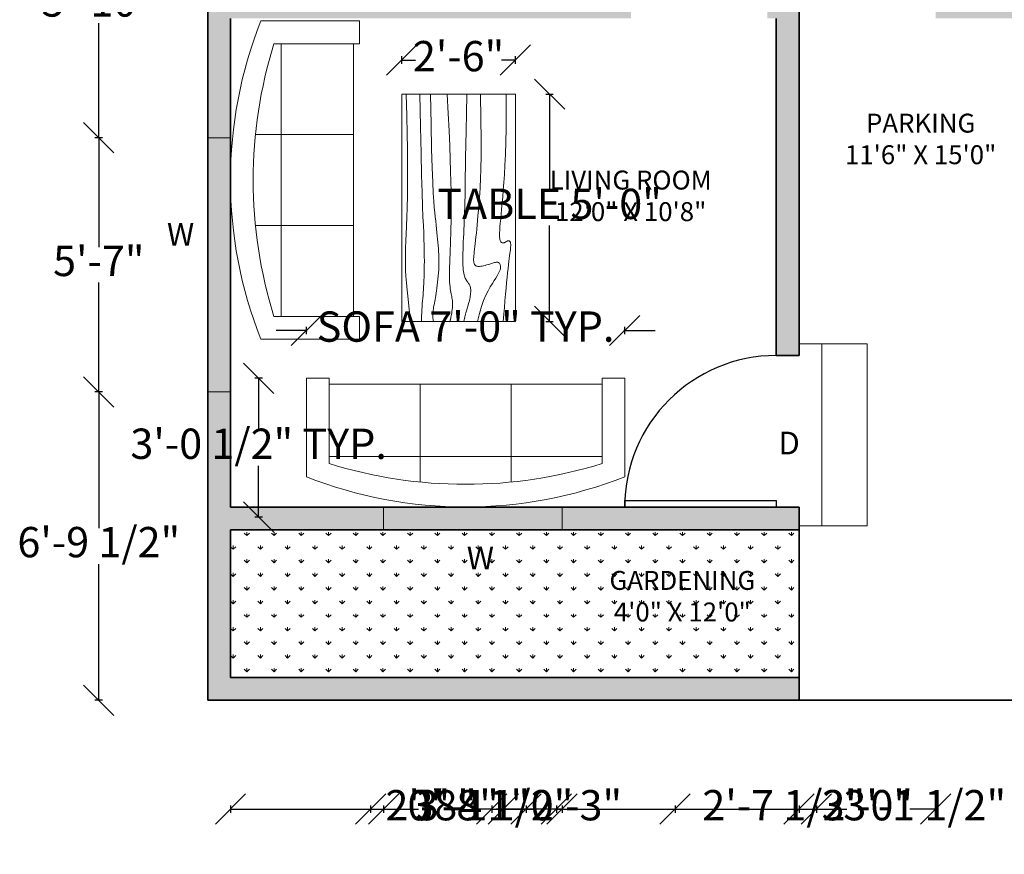
# Model space of a CAD drawing. Units: inches. Extents: x 2247 to 2713, y 588 to 1209.
# Tile 1 of 5: x 2314 to 2574, y 588 to 808. Entities that reach past the tile are written whole.
import ezdxf

# ---------------------------------------------------------------- set-up
doc = ezdxf.new("R2010")
doc.units = ezdxf.units.IN
for name, color, linetype, lineweight in [('A-ANNO-DIMS', 2, 'Continuous', 18), ('A-ANNO-TEXT', 7, 'Continuous', 18), ('A-AREA-IDEN', 7, 'Continuous', 25), ('A-DOOR', 3, 'Continuous', 25), ('A-FLOR-STRS', 7, 'Continuous', 18), ('A-FURN', 8, 'Continuous', 18), ('A-GLAZ', 4, 'Continuous', 18), ('A-GLAZ-PATT', 7, 'Continuous', 13), ('A-WALL', 7, 'Continuous', 35), ('A-WALL-PATT', 4, 'Continuous', 13)]:
    doc.layers.add(name, color=color, linetype=linetype, lineweight=lineweight)
doc.layers.add('L-PLNT-PATT', color=116, linetype='Continuous', lineweight=13, true_color=0x136734)
doc.styles.get("Standard").update_dxf_attribs({"font": 'arial.ttf'})
doc.dimstyles.new('ISO-25', dxfattribs={"dimtxt": 8, "dimasz": 8, "dimexe": 1, "dimexo": 1, "dimtad": 0, "dimtih": 1, "dimtoh": 1, "dimlunit": 3, "dimtxsty": 'Standard', "dimblk": 'OBLIQUE', "dimcen": 2.5, "dimadec": 0, "dimazin": 0, "dimtfac": 1, "dimtmove": 0, "dimatfit": 3, "dimfxl": 1, "dimfxlon": 1, "dimarcsym": 0})

# ---------------------------------------------------------------- blocks, each defined once
blk = doc.blocks.new('*U3')
for p, q in [((0, 0), (0, -6)), ((40, 0), (40, -6))]:
    blk.add_line(p, q)
blk.add_lwpolyline([(0, 0), (0, 40), (1.75, 40), (1.75, 0)], close=True)
blk.add_arc((0, 0), 40, 0, 90)
blk = doc.blocks.new('Sofa - Roundback 7 ft.')
for p, q in [((-12.00002, -32.4421), (-12.00003, -6.5971)), ((11.99997, -32.4421), (11.99998, -6.5971)), ((-36.000027, -34), (-36.000027, -11.4696)), ((35.99998, -34), (35.99998, -11.4696)), ((-35.999844, -13.3819), (35.9998, -13.3819)), ((-36.000027, -32.4421), (35.99998, -32.4421))]:
    blk.add_line(p, q)
for points in [[(-36.000027, -34), (-42.000027, -34), (-42.000027, -8)], [(41.99998, -8), (41.99998, -34), (35.99998, -34)]]:
    blk.add_lwpolyline(points)
for centre, radius, start, end in [((0, -114.25), 114.25, 68.43141, 111.5686), ((-0.00001, -127.1968), 121.1968, 72.72033, 107.2797)]:
    blk.add_arc(centre, radius, start, end)
blk = doc.blocks.new('Table - Rectangular Woodgrain 60 x 30 in.')
for p, q in [((0, 0), (0, -30)), ((60, 0), (0, 0)), ((60, -30), (60, 0)), ((0, -30), (60, -30))]:
    blk.add_line(p, q)
for points in [[(0, -2.4), (4.8155, -2.418), (9.0302, -2.4688), (12.709, -2.5477), (15.9167, -2.65), (18.7181, -2.7711), (21.1781, -2.9063), (23.3616, -3.0508), (25.3333, -3.2), (27.1477, -3.3495), (28.8172, -3.4958), (30.3437, -3.636), (31.7291, -3.7667), (32.9756, -3.8849), (34.0849, -3.9875), (35.059, -4.0714), (35.9, -4.1334), (36.6114, -4.1711), (37.2041, -4.1854), (37.6906, -4.1779), (38.0833, -4.15), (38.3948, -4.1034), (38.6375, -4.0396), (38.8239, -3.9602), (38.9666, -3.8667), (39.0764, -3.7608), (39.1573, -3.6448), (39.2116, -3.521), (39.2416, -3.3917), (39.2498, -3.2593), (39.2385, -3.1261), (39.21, -2.9944), (39.1666, -2.8667), (39.111, -2.7447), (39.0468, -2.6281), (38.978, -2.5163), (38.9083, -2.4083), (38.8418, -2.3035), (38.7823, -2.201), (38.7337, -2.1001), (38.7, -2), (38.6844, -1.9003), (38.6875, -1.8021), (38.7094, -1.707), (38.75, -1.6167), (38.8094, -1.5326), (38.8875, -1.4563), (38.9844, -1.3893), (39.1, -1.3333), (39.2351, -1.2896), (39.3937, -1.2583), (39.5804, -1.2396), (39.8, -1.2333), (40.057, -1.2396), (40.3562, -1.2583), (40.7023, -1.2896), (41.1, -1.3333), (41.5547, -1.3895), (42.0755, -1.4573), (42.6721, -1.5361), (43.3542, -1.625), (44.1316, -1.7233), (45.014, -1.8302), (46.0114, -1.9449), (47.1333, -2.0667), (48.3862, -2.1947), (49.7625, -2.3281), (51.2513, -2.4663), (52.8416, -2.6083), (54.5226, -2.7535), (56.2833, -2.9011), (58.1127, -3.0501), (60, -3.2)], [(0, -9.2), (6.5759, -9.0858), (11.9385, -9.0365), (16.2527, -9.0418), (19.6833, -9.0917), (22.3952, -9.1759), (24.5531, -9.2844), (26.322, -9.4069), (27.8666, -9.5333), (29.3241, -9.6553), (30.7203, -9.7719), (32.0532, -9.8837), (33.3208, -9.9917), (34.5213, -10.0965), (35.6526, -10.199), (36.7128, -10.2999), (37.7, -10.4), (38.6129, -10.4996), (39.4531, -10.5969), (40.223, -10.6895), (40.925, -10.775), (41.5613, -10.8512), (42.1344, -10.9156), (42.6465, -10.966), (43.1, -11), (43.4976, -11.0158), (43.8437, -11.0136), (44.143, -10.9942), (44.4, -10.9583), (44.6195, -10.9069), (44.8062, -10.8406), (44.9648, -10.7603), (45.1, -10.6667), (45.2155, -10.5598), (45.3114, -10.4365), (45.3871, -10.2929), (45.4416, -10.125), (45.4743, -9.929), (45.4844, -9.7011), (45.4709, -9.4371), (45.4333, -9.1333), (45.3716, -8.7883), (45.2896, -8.4104), (45.1919, -8.0107), (45.0833, -7.6), (44.9685, -7.1893), (44.8521, -6.7896), (44.7388, -6.4117), (44.6333, -6.0667), (44.54, -5.7628), (44.4614, -5.4979), (44.4001, -5.2675), (44.3583, -5.0667), (44.3384, -4.8909), (44.3427, -4.7354), (44.3736, -4.5956), (44.4333, -4.4667), (44.5236, -4.3453), (44.6427, -4.2333), (44.7884, -4.1339), (44.9583, -4.05), (45.1501, -3.9849), (45.3614, -3.9417), (45.59, -3.9234), (45.8333, -3.9333), (46.0915, -3.9749), (46.3734, -4.0531), (46.6906, -4.1736), (47.0542, -4.3417), (47.4756, -4.5629), (47.9661, -4.8427), (48.5372, -5.1866), (49.2, -5.6), (49.9676, -6.0844), (50.8594, -6.625), (51.8965, -7.2031), (53.1, -7.8), (54.491, -8.3969), (56.0906, -8.975), (57.9199, -9.5156), (60, -10)], [(0, -12.8), (5.1847, -12.9322), (9.6213, -13.0323), (13.3963, -13.1059), (16.5958, -13.1583), (19.3063, -13.1952), (21.614, -13.2219), (23.6054, -13.2439), (25.3666, -13.2667), (26.9728, -13.2947), (28.4531, -13.3281), (29.8256, -13.3663), (31.1083, -13.4083), (32.3191, -13.4535), (33.476, -13.501), (34.597, -13.5501), (35.7, -13.6), (36.7984, -13.6497), (37.8875, -13.6979), (38.9578, -13.743), (40, -13.7833), (41.0047, -13.8174), (41.9625, -13.8438), (42.864, -13.8607), (43.7, -13.8667), (44.4631, -13.8604), (45.1552, -13.8417), (45.7801, -13.8104), (46.3416, -13.7667), (46.8439, -13.7104), (47.2906, -13.6417), (47.6858, -13.5604), (48.0333, -13.4667), (48.3375, -13.3608), (48.6042, -13.2448), (48.8396, -13.121), (49.05, -12.9917), (49.2417, -12.8593), (49.4208, -12.7261), (49.5937, -12.5944), (49.7667, -12.4667), (49.9452, -12.3451), (50.1323, -12.2313), (50.3303, -12.1268), (50.5416, -12.0333), (50.7686, -11.9524), (51.0135, -11.8854), (51.2788, -11.8341), (51.5666, -11.8), (51.8785, -11.7843), (52.2116, -11.7865), (52.562, -11.8059), (52.926, -11.8417), (53.2998, -11.8931), (53.6795, -11.9594), (54.0614, -12.0397), (54.4416, -12.1333), (54.8223, -12.2401), (55.2293, -12.3625), (55.6942, -12.5037), (56.2489, -12.6667), (56.9251, -12.8547), (57.7545, -13.0708), (58.7689, -13.3182), (60, -13.6)], [(0, -18), (5.124, -17.7273), (9.6609, -17.5057), (13.6705, -17.3303), (17.2125, -17.1958), (20.3467, -17.0973), (23.1328, -17.0297), (25.6307, -16.9878), (27.9, -16.9667), (29.9928, -16.9617), (31.9302, -16.9703), (33.7254, -16.9907), (35.3917, -17.0208), (36.9423, -17.0588), (38.3906, -17.1026), (39.7499, -17.1503), (41.0333, -17.2), (42.2519, -17.2496), (43.4073, -17.2969), (44.4986, -17.3395), (45.525, -17.375), (46.4858, -17.4012), (47.3802, -17.4156), (48.2074, -17.416), (48.9667, -17.4), (49.6583, -17.3662), (50.2872, -17.3167), (50.8595, -17.2547), (51.3812, -17.1833), (51.8584, -17.1057), (52.2971, -17.025), (52.7034, -16.9443), (53.0833, -16.8667), (53.443, -16.7951), (53.789, -16.7313), (54.128, -16.6768), (54.4666, -16.6334), (54.8115, -16.6024), (55.1693, -16.5854), (55.5465, -16.5841), (55.95, -16.6), (56.3828, -16.6337), (56.8346, -16.6823), (57.2915, -16.7418), (57.7396, -16.8084), (58.165, -16.878), (58.5539, -16.9469), (58.8924, -17.0111), (59.1666, -17.0667), (59.3679, -17.1107), (59.5078, -17.1438), (59.6032, -17.1675), (59.6708, -17.1833), (59.7275, -17.193), (59.7901, -17.1979), (59.8753, -17.1998), (60, -17.2)], [(0, -22.4), (8.0098, -22.2501), (14.4094, -22.1011), (19.4168, -21.9535), (23.25, -21.8083), (26.1269, -21.6663), (28.2656, -21.5281), (29.884, -21.3947), (31.2, -21.2667), (32.3967, -21.1448), (33.5172, -21.0292), (34.5697, -20.9198), (35.5625, -20.8167), (36.5037, -20.7198), (37.4015, -20.6292), (38.2642, -20.5448), (39.1, -20.4667), (39.9164, -20.3951), (40.7187, -20.3313), (41.5117, -20.2768), (42.3, -20.2333), (43.0883, -20.2024), (43.8812, -20.1854), (44.6836, -20.1841), (45.5, -20.2), (46.3328, -20.234), (47.1747, -20.2844), (48.0163, -20.3488), (48.8479, -20.425), (49.66, -20.5106), (50.4429, -20.6031), (51.1872, -20.7004), (51.8833, -20.8), (52.5246, -20.8999), (53.1166, -20.9995), (53.6681, -21.0983), (54.1875, -21.1958), (54.6834, -21.2919), (55.1646, -21.3859), (55.6394, -21.4777), (56.1167, -21.5667), (56.6028, -21.6515), (57.0961, -21.7266), (57.5929, -21.7852), (58.0896, -21.8208), (58.5823, -21.8268), (59.0674, -21.7964), (59.5412, -21.723), (60, -21.6)], [(0, -25.2), (8.6355, -25.0504), (15.7026, -24.9031), (21.4049, -24.7606), (25.9458, -24.625), (29.529, -24.4988), (32.3578, -24.3844), (34.6359, -24.284), (36.5667, -24.2), (38.3213, -24.1341), (39.9417, -24.0854), (41.437, -24.0523), (42.8167, -24.0333), (44.0901, -24.0268), (45.2667, -24.0313), (46.3557, -24.0451), (47.3667, -24.0667), (48.309, -24.0947), (49.1928, -24.1287), (50.0284, -24.168), (50.826, -24.2125), (51.5959, -24.2617), (52.3483, -24.3151), (53.0935, -24.3725), (53.8417, -24.4334), (54.6009, -24.497), (55.3699, -24.561), (56.1454, -24.6226), (56.9239, -24.6792), (57.7021, -24.7279), (58.4764, -24.7662), (59.2435, -24.7911), (60, -24.8)], [(0, -28.8), (5.6867, -28.6681), (10.45, -28.5698), (14.407, -28.5012), (17.675, -28.4584), (20.3711, -28.4374), (22.6125, -28.4344), (24.5164, -28.4455), (26.2, -28.4667), (27.762, -28.4947), (29.2276, -28.5281), (30.6033, -28.5663), (31.8958, -28.6084), (33.1118, -28.6535), (34.2578, -28.7011), (35.3405, -28.7501), (36.3666, -28.8), (37.3443, -28.8497), (38.288, -28.8974), (39.2137, -28.9412), (40.1375, -28.9792), (41.0753, -29.0093), (42.0432, -29.0297), (43.0572, -29.0384), (44.1333, -29.0333), (45.2936, -29.0114), (46.5843, -28.9641), (48.0579, -28.8816), (49.7666, -28.7542), (51.7629, -28.5721), (54.0989, -28.3255), (56.8272, -28.0048), (60, -27.6)]]:
    blk.add_lwpolyline(points)
blk = doc.blocks.new('_Oblique')
at = {"color": 0, "linetype": 'ByBlock', "lineweight": -2}
blk.add_line((-0.5, -0.5), (0.5, 0.5), dxfattribs=at)
blk = doc.blocks.new('*D19')
at = {"layer": 'A-ANNO-DIMS', "color": 0, "lineweight": -2, "transparency": 16777216}
for p, q in [((2390.1, 725.88), (2382.1, 725.88)), ((2390.1, 724.88), (2390.1, 726.88)), ((2390.1, 725.88), (2390.34, 725.88)), ((2474.1, 725.88), (2473.85, 725.88)), ((2474.1, 724.88), (2474.1, 726.88)), ((2474.1, 725.88), (2482.1, 725.88))]:
    blk.add_line(p, q, dxfattribs=at)
at = {"layer": 'Defpoints', "color": 0, "transparency": 16777216}
for p in [(2390.1, 725.88), (2390.1, 713.28), (2474.1, 713.28)]:
    blk.add_point(p, dxfattribs=at)
at = {"layer": 'A-ANNO-DIMS', "color": 0, "lineweight": -2, "transparency": 16777216, "xscale": 8, "yscale": 8, "zscale": 8}
blk.add_blockref('_Oblique', (2390.1, 725.88), dxfattribs=at)
at = {"layer": 'A-ANNO-DIMS', "color": 0, "lineweight": -2, "transparency": 16777216, "xscale": 8, "yscale": 8, "zscale": 8, "rotation": 180}
blk.add_blockref('_Oblique', (2474.1, 725.88), dxfattribs=at)
at = {"layer": 'A-ANNO-DIMS', "color": 0, "transparency": 16777216, "insert": (2432.1, 725.88), "char_height": 8, "attachment_point": 5}
blk.add_mtext('SOFA 7\'-0" TYP.', dxfattribs=at)
blk = doc.blocks.new('*D20')
at = {"layer": 'A-ANNO-DIMS', "color": 0, "lineweight": -2, "transparency": 16777216}
for p, q in [((2378.5, 713.28), (2376.5, 713.28)), ((2377.5, 713.28), (2377.5, 699.71)), ((2377.5, 676.61), (2377.5, 690.18)), ((2378.5, 676.61), (2376.5, 676.61))]:
    blk.add_line(p, q, dxfattribs=at)
at = {"layer": 'Defpoints', "color": 0, "transparency": 16777216}
for p in [(2390.1, 713.28), (2377.5, 676.61), (2390.1, 676.61)]:
    blk.add_point(p, dxfattribs=at)
at = {"layer": 'A-ANNO-DIMS', "color": 0, "lineweight": -2, "transparency": 16777216, "xscale": 8, "yscale": 8, "zscale": 8}
for p, rotation in [((2377.5, 713.28), 90), ((2377.5, 676.61), 270)]:
    blk.add_blockref('_Oblique', p, dxfattribs=dict(at, rotation=rotation))
at = {"layer": 'A-ANNO-DIMS', "color": 0, "transparency": 16777216, "insert": (2377.5, 694.95), "char_height": 8, "attachment_point": 5}
blk.add_mtext('3\'-0 1/2" TYP.', dxfattribs=at)
blk = doc.blocks.new('*D21')
at = {"layer": 'A-ANNO-DIMS', "color": 0, "lineweight": -2, "transparency": 16777216}
for p, q in [((2453.25, 788.27), (2455.25, 788.27)), ((2454.25, 788.27), (2454.25, 762.98)), ((2454.25, 728.27), (2454.25, 753.56)), ((2453.25, 728.27), (2455.25, 728.27))]:
    blk.add_line(p, q, dxfattribs=at)
at = {"layer": 'Defpoints', "color": 0, "transparency": 16777216}
for p in [(2445.25, 788.27), (2445.25, 728.27), (2454.25, 728.27)]:
    blk.add_point(p, dxfattribs=at)
at = {"layer": 'A-ANNO-DIMS', "color": 0, "lineweight": -2, "transparency": 16777216, "xscale": 8, "yscale": 8, "zscale": 8}
for p, rotation in [((2454.25, 788.27), 90), ((2454.25, 728.27), 270)]:
    blk.add_blockref('_Oblique', p, dxfattribs=dict(at, rotation=rotation))
at = {"layer": 'A-ANNO-DIMS', "color": 0, "transparency": 16777216, "insert": (2454.25, 758.27), "char_height": 8, "attachment_point": 5}
blk.add_mtext('TABLE 5\'-0"', dxfattribs=at)
blk = doc.blocks.new('*D22')
at = {"layer": 'A-ANNO-DIMS', "color": 0, "lineweight": -2, "transparency": 16777216}
for p, q in [((2415.25, 796.27), (2415.25, 798.27)), ((2445.25, 796.27), (2445.25, 798.27)), ((2415.25, 797.27), (2418.92, 797.27)), ((2445.25, 797.27), (2441.57, 797.27))]:
    blk.add_line(p, q, dxfattribs=at)
at = {"layer": 'Defpoints', "color": 0, "transparency": 16777216}
for p in [(2445.25, 797.27), (2415.25, 788.27), (2445.25, 788.27)]:
    blk.add_point(p, dxfattribs=at)
at = {"layer": 'A-ANNO-DIMS', "color": 0, "lineweight": -2, "transparency": 16777216, "xscale": 8, "yscale": 8, "zscale": 8, "rotation": 180}
blk.add_blockref('_Oblique', (2415.25, 797.27), dxfattribs=at)
at = {"layer": 'A-ANNO-DIMS', "color": 0, "lineweight": -2, "transparency": 16777216, "xscale": 8, "yscale": 8, "zscale": 8}
blk.add_blockref('_Oblique', (2445.25, 797.27), dxfattribs=at)
at = {"layer": 'A-ANNO-DIMS', "color": 0, "transparency": 16777216, "insert": (2430.25, 797.27), "char_height": 8, "attachment_point": 5}
blk.add_mtext('2\'-6"', dxfattribs=at)
blk = doc.blocks.new('*D25')
at = {"layer": 'A-ANNO-DIMS', "color": 0, "lineweight": -2, "transparency": 16777216}
for p, q in [((2691.83, 719.28), (2693.83, 719.28)), ((2692.83, 719.28), (2692.83, 703.99)), ((2692.83, 679.28), (2692.83, 694.57)), ((2691.83, 679.28), (2693.83, 679.28))]:
    blk.add_line(p, q, dxfattribs=at)
at = {"layer": 'Defpoints', "color": 0, "transparency": 16777216}
for p in [(2520.08, 719.28), (2692.83, 719.28), (2520.08, 679.28)]:
    blk.add_point(p, dxfattribs=at)
at = {"layer": 'A-ANNO-DIMS', "color": 0, "lineweight": -2, "transparency": 16777216, "xscale": 8, "yscale": 8, "zscale": 8}
for p, rotation in [((2692.83, 719.28), 90), ((2692.83, 679.28), 270)]:
    blk.add_blockref('_Oblique', p, dxfattribs=dict(at, rotation=rotation))
at = {"layer": 'A-ANNO-DIMS', "color": 0, "transparency": 16777216, "insert": (2692.83, 699.28), "char_height": 8, "attachment_point": 5}
blk.add_mtext('3\'-4"', dxfattribs=at)
blk = doc.blocks.new('*D26')
at = {"layer": 'A-ANNO-DIMS', "color": 0, "lineweight": -2, "transparency": 16777216}
for p, q in [((2520.08, 600.53), (2520.08, 598.53)), ((2556.08, 600.53), (2556.08, 598.53)), ((2520.08, 599.53), (2526.82, 599.53)), ((2556.08, 599.53), (2549.33, 599.53))]:
    blk.add_line(p, q, dxfattribs=at)
at = {"layer": 'Defpoints', "color": 0, "transparency": 16777216}
for p in [(2520.08, 808.28), (2556.08, 808.28), (2556.08, 599.53)]:
    blk.add_point(p, dxfattribs=at)
at = {"layer": 'A-ANNO-DIMS', "color": 0, "lineweight": -2, "transparency": 16777216, "xscale": 8, "yscale": 8, "zscale": 8, "rotation": 180}
blk.add_blockref('_Oblique', (2520.08, 599.53), dxfattribs=at)
at = {"layer": 'A-ANNO-DIMS', "color": 0, "lineweight": -2, "transparency": 16777216, "xscale": 8, "yscale": 8, "zscale": 8}
blk.add_blockref('_Oblique', (2556.08, 599.53), dxfattribs=at)
at = {"layer": 'A-ANNO-DIMS', "color": 0, "transparency": 16777216, "insert": (2538.08, 599.53), "char_height": 8, "attachment_point": 5}
blk.add_mtext('3\'-0"', dxfattribs=at)
blk = doc.blocks.new('*D27')
at = {"layer": 'A-ANNO-DIMS', "color": 0, "lineweight": -2, "transparency": 16777216}
for p, q in [((2407.02, 600.53), (2407.02, 598.53)), ((2439.02, 600.53), (2439.02, 598.53)), ((2407.02, 599.53), (2411.7, 599.53)), ((2439.02, 599.53), (2434.35, 599.53))]:
    blk.add_line(p, q, dxfattribs=at)
at = {"layer": 'Defpoints', "color": 0, "transparency": 16777216}
for p in [(2407.02, 1108.28), (2439.02, 1108.28), (2439.02, 599.53)]:
    blk.add_point(p, dxfattribs=at)
at = {"layer": 'A-ANNO-DIMS', "color": 0, "lineweight": -2, "transparency": 16777216, "xscale": 8, "yscale": 8, "zscale": 8, "rotation": 180}
blk.add_blockref('_Oblique', (2407.02, 599.53), dxfattribs=at)
at = {"layer": 'A-ANNO-DIMS', "color": 0, "lineweight": -2, "transparency": 16777216, "xscale": 8, "yscale": 8, "zscale": 8}
blk.add_blockref('_Oblique', (2439.02, 599.53), dxfattribs=at)
at = {"layer": 'A-ANNO-DIMS', "color": 0, "transparency": 16777216, "insert": (2423.02, 599.53), "char_height": 8, "attachment_point": 5}
blk.add_mtext('2\'-8"', dxfattribs=at)
blk = doc.blocks.new('*D33')
at = {"layer": 'A-ANNO-DIMS', "color": 0, "lineweight": -2, "transparency": 16777216}
for p, q in [((2336.33, 709.67), (2334.33, 709.67)), ((2335.33, 709.67), (2335.33, 673.74)), ((2335.33, 628.28), (2335.33, 664.22)), ((2336.33, 628.28), (2334.33, 628.28))]:
    blk.add_line(p, q, dxfattribs=at)
at = {"layer": 'Defpoints', "color": 0, "transparency": 16777216}
for p in [(2335.33, 709.67), (2364.08, 709.67), (2364.08, 628.28)]:
    blk.add_point(p, dxfattribs=at)
at = {"layer": 'A-ANNO-DIMS', "color": 0, "lineweight": -2, "transparency": 16777216, "xscale": 8, "yscale": 8, "zscale": 8}
for p, rotation in [((2335.33, 709.67), 90), ((2335.33, 628.28), 270)]:
    blk.add_blockref('_Oblique', p, dxfattribs=dict(at, rotation=rotation))
at = {"layer": 'A-ANNO-DIMS', "color": 0, "transparency": 16777216, "insert": (2335.33, 668.98), "char_height": 8, "attachment_point": 5}
blk.add_mtext('6\'-9 1/2"', dxfattribs=at)
blk = doc.blocks.new('*D34')
at = {"layer": 'A-ANNO-DIMS', "color": 0, "lineweight": -2, "transparency": 16777216}
for p, q in [((2336.33, 776.75), (2334.33, 776.75)), ((2335.33, 776.75), (2335.33, 747.9)), ((2335.33, 709.67), (2335.33, 738.52)), ((2336.33, 709.67), (2334.33, 709.67))]:
    blk.add_line(p, q, dxfattribs=at)
at = {"layer": 'Defpoints', "color": 0, "transparency": 16777216}
for p in [(2335.33, 776.75), (2364.08, 776.75), (2364.08, 709.67)]:
    blk.add_point(p, dxfattribs=at)
at = {"layer": 'A-ANNO-DIMS', "color": 0, "lineweight": -2, "transparency": 16777216, "xscale": 8, "yscale": 8, "zscale": 8}
for p, rotation in [((2335.33, 776.75), 90), ((2335.33, 709.67), 270)]:
    blk.add_blockref('_Oblique', p, dxfattribs=dict(at, rotation=rotation))
at = {"layer": 'A-ANNO-DIMS', "color": 0, "transparency": 16777216, "insert": (2335.33, 743.21), "char_height": 8, "attachment_point": 5}
blk.add_mtext('5\'-7"', dxfattribs=at)
blk = doc.blocks.new('*D35')
at = {"layer": 'A-ANNO-DIMS', "color": 0, "lineweight": -2, "transparency": 16777216}
for p, q in [((2336.33, 846.66), (2334.33, 846.66)), ((2335.33, 846.66), (2335.33, 816.41)), ((2335.33, 776.75), (2335.33, 806.99)), ((2336.33, 776.75), (2334.33, 776.75))]:
    blk.add_line(p, q, dxfattribs=at)
at = {"layer": 'Defpoints', "color": 0, "transparency": 16777216}
for p in [(2335.33, 846.66), (2364.08, 846.66), (2364.08, 776.75)]:
    blk.add_point(p, dxfattribs=at)
at = {"layer": 'A-ANNO-DIMS', "color": 0, "lineweight": -2, "transparency": 16777216, "xscale": 8, "yscale": 8, "zscale": 8}
for p, rotation in [((2335.33, 846.66), 90), ((2335.33, 776.75), 270)]:
    blk.add_blockref('_Oblique', p, dxfattribs=dict(at, rotation=rotation))
at = {"layer": 'A-ANNO-DIMS', "color": 0, "transparency": 16777216, "insert": (2335.33, 811.7), "char_height": 8, "attachment_point": 5}
blk.add_mtext('5\'-10"', dxfattribs=at)
blk = doc.blocks.new('*D45')
at = {"layer": 'A-ANNO-DIMS', "color": 0, "lineweight": -2, "transparency": 16777216}
for p, q in [((2456.06, 600.53), (2456.06, 598.53)), ((2487.37, 600.53), (2487.37, 598.53)), ((2456.06, 599.53), (2487.37, 599.53)), ((2487.37, 599.53), (2495.37, 599.53))]:
    blk.add_line(p, q, dxfattribs=at)
at = {"layer": 'Defpoints', "color": 0, "transparency": 16777216}
for p in [(2456.06, 1108.28), (2487.37, 1108.28), (2487.37, 599.53)]:
    blk.add_point(p, dxfattribs=at)
at = {"layer": 'A-ANNO-DIMS', "color": 0, "lineweight": -2, "transparency": 16777216, "xscale": 8, "yscale": 8, "zscale": 8, "rotation": 180}
blk.add_blockref('_Oblique', (2456.06, 599.53), dxfattribs=at)
at = {"layer": 'A-ANNO-DIMS', "color": 0, "lineweight": -2, "transparency": 16777216, "xscale": 8, "yscale": 8, "zscale": 8}
blk.add_blockref('_Oblique', (2487.37, 599.53), dxfattribs=at)
at = {"layer": 'A-ANNO-DIMS', "color": 0, "transparency": 16777216, "insert": (2516.02, 599.53), "char_height": 8, "attachment_point": 5}
blk.add_mtext('2\'-7 1/2"', dxfattribs=at)
blk = doc.blocks.new('*D47')
at = {"layer": 'A-ANNO-DIMS', "color": 0, "lineweight": -2, "transparency": 16777216}
for p, q in [((2487.37, 600.53), (2487.37, 598.53)), ((2524.66, 600.53), (2524.66, 598.53)), ((2487.37, 599.53), (2524.66, 599.53)), ((2524.66, 599.53), (2532.66, 599.53))]:
    blk.add_line(p, q, dxfattribs=at)
at = {"layer": 'Defpoints', "color": 0, "transparency": 16777216}
for p in [(2487.37, 1108.28), (2524.66, 1108.28), (2524.66, 599.53)]:
    blk.add_point(p, dxfattribs=at)
at = {"layer": 'A-ANNO-DIMS', "color": 0, "lineweight": -2, "transparency": 16777216, "xscale": 8, "yscale": 8, "zscale": 8, "rotation": 180}
blk.add_blockref('_Oblique', (2487.37, 599.53), dxfattribs=at)
at = {"layer": 'A-ANNO-DIMS', "color": 0, "lineweight": -2, "transparency": 16777216, "xscale": 8, "yscale": 8, "zscale": 8}
blk.add_blockref('_Oblique', (2524.66, 599.53), dxfattribs=at)
at = {"layer": 'A-ANNO-DIMS', "color": 0, "transparency": 16777216, "insert": (2553.24, 599.53), "char_height": 8, "attachment_point": 5}
blk.add_mtext('3\'-1 1/2"', dxfattribs=at)
blk = doc.blocks.new('*D48')
at = {"layer": 'A-ANNO-DIMS', "color": 0, "lineweight": -2, "transparency": 16777216}
for p, q in [((2448.08, 600.53), (2448.08, 598.53)), ((2456.06, 600.53), (2456.06, 598.53)), ((2448.08, 599.53), (2440.08, 599.53)), ((2456.06, 599.53), (2448.08, 599.53))]:
    blk.add_line(p, q, dxfattribs=at)
at = {"layer": 'Defpoints', "color": 0, "transparency": 16777216}
for p in [(2448.08, 1114.28), (2456.06, 1114.28), (2448.08, 599.53)]:
    blk.add_point(p, dxfattribs=at)
at = {"layer": 'A-ANNO-DIMS', "color": 0, "lineweight": -2, "transparency": 16777216, "xscale": 8, "yscale": 8, "zscale": 8, "rotation": 180}
blk.add_blockref('_Oblique', (2448.08, 599.53), dxfattribs=at)
at = {"layer": 'A-ANNO-DIMS', "color": 0, "lineweight": -2, "transparency": 16777216, "xscale": 8, "yscale": 8, "zscale": 8}
blk.add_blockref('_Oblique', (2456.06, 599.53), dxfattribs=at)
at = {"layer": 'A-ANNO-DIMS', "color": 0, "transparency": 16777216, "insert": (2428.82, 599.53), "char_height": 8, "attachment_point": 5}
blk.add_mtext('0\'-8"', dxfattribs=at)
blk = doc.blocks.new('*D51')
at = {"layer": 'A-ANNO-DIMS', "color": 0, "lineweight": -2, "transparency": 16777216}
for p, q in [((2410.48, 600.53), (2410.48, 598.53)), ((2457.58, 600.53), (2457.58, 598.53)), ((2410.48, 599.53), (2419.67, 599.53)), ((2457.58, 599.53), (2448.39, 599.53))]:
    blk.add_line(p, q, dxfattribs=at)
at = {"layer": 'Defpoints', "color": 0, "transparency": 16777216}
for p in [(2410.48, 673.28), (2457.58, 673.28), (2457.58, 599.53)]:
    blk.add_point(p, dxfattribs=at)
at = {"layer": 'A-ANNO-DIMS', "color": 0, "lineweight": -2, "transparency": 16777216, "xscale": 8, "yscale": 8, "zscale": 8, "rotation": 180}
blk.add_blockref('_Oblique', (2410.48, 599.53), dxfattribs=at)
at = {"layer": 'A-ANNO-DIMS', "color": 0, "lineweight": -2, "transparency": 16777216, "xscale": 8, "yscale": 8, "zscale": 8}
blk.add_blockref('_Oblique', (2457.58, 599.53), dxfattribs=at)
at = {"layer": 'A-ANNO-DIMS', "color": 0, "transparency": 16777216, "insert": (2434.03, 599.53), "char_height": 8, "attachment_point": 5}
blk.add_mtext('3\'-11"', dxfattribs=at)
blk = doc.blocks.new('*D52')
at = {"layer": 'A-ANNO-DIMS', "color": 0, "lineweight": -2, "transparency": 16777216}
for p, q in [((2370.08, 600.53), (2370.08, 598.53)), ((2410.48, 600.53), (2410.48, 598.53)), ((2370.08, 599.53), (2410.48, 599.53)), ((2410.48, 599.53), (2418.48, 599.53))]:
    blk.add_line(p, q, dxfattribs=at)
at = {"layer": 'Defpoints', "color": 0, "transparency": 16777216}
for p in [(2370.08, 673.28), (2410.48, 673.28), (2410.48, 599.53)]:
    blk.add_point(p, dxfattribs=at)
at = {"layer": 'A-ANNO-DIMS', "color": 0, "lineweight": -2, "transparency": 16777216, "xscale": 8, "yscale": 8, "zscale": 8, "rotation": 180}
blk.add_blockref('_Oblique', (2370.08, 599.53), dxfattribs=at)
at = {"layer": 'A-ANNO-DIMS', "color": 0, "lineweight": -2, "transparency": 16777216, "xscale": 8, "yscale": 8, "zscale": 8}
blk.add_blockref('_Oblique', (2410.48, 599.53), dxfattribs=at)
at = {"layer": 'A-ANNO-DIMS', "color": 0, "transparency": 16777216, "insert": (2439.05, 599.53), "char_height": 8, "attachment_point": 5}
blk.add_mtext('3\'-4 1/2"', dxfattribs=at)
blk = doc.blocks.new('*D55')
at = {"layer": 'A-ANNO-DIMS', "color": 0, "lineweight": -2, "transparency": 16777216}
for p, q in [((2439.02, 600.53), (2439.02, 598.53)), ((2442.08, 600.53), (2442.08, 598.53)), ((2439.02, 599.53), (2442.08, 599.53)), ((2442.08, 599.53), (2450.08, 599.53))]:
    blk.add_line(p, q, dxfattribs=at)
at = {"layer": 'Defpoints', "color": 0, "transparency": 16777216}
for p in [(2442.08, 1114.28), (2439.02, 1108.28), (2442.08, 599.53)]:
    blk.add_point(p, dxfattribs=at)
at = {"layer": 'A-ANNO-DIMS', "color": 0, "lineweight": -2, "transparency": 16777216, "xscale": 8, "yscale": 8, "zscale": 8, "rotation": 180}
blk.add_blockref('_Oblique', (2439.02, 599.53), dxfattribs=at)
at = {"layer": 'A-ANNO-DIMS', "color": 0, "lineweight": -2, "transparency": 16777216, "xscale": 8, "yscale": 8, "zscale": 8}
blk.add_blockref('_Oblique', (2442.08, 599.53), dxfattribs=at)
at = {"layer": 'A-ANNO-DIMS', "color": 0, "transparency": 16777216, "insert": (2461.33, 599.53), "char_height": 8, "attachment_point": 5}
blk.add_mtext('0\'-3"', dxfattribs=at)

msp = doc.modelspace()

# ---------------------------------------------------------------- hatches: boundary and pattern name
at = {"layer": 'A-GLAZ-PATT'}
h = msp.add_hatch(color=256, dxfattribs=at)
h.dxf.hatch_style = 1
h.paths.add_polyline_path([(2423.716, 1168.28), (2380.833, 1168.28), (2380.833, 1162.28), (2423.716, 1162.28)])
h.paths.add_polyline_path([(2487.371, 1114.28), (2456.056, 1114.28), (2456.056, 1108.28), (2487.371, 1108.28)])
h.paths.add_polyline_path([(2560.507, 1114.28), (2524.66, 1114.28), (2524.66, 1108.28), (2560.507, 1108.28)])
h.paths.add_polyline_path([(2639.393, 1168.28), (2604.041, 1168.28), (2604.041, 1162.28), (2639.393, 1162.28)])
h.paths.add_polyline_path([(2370.076, 1094.128), (2364.076, 1094.128), (2364.076, 1054.172), (2370.076, 1054.172), (2370.076, 1068.35)])
h.paths.add_polyline_path([(2370.076, 990.686), (2364.076, 990.686), (2364.076, 950.99), (2370.076, 950.99)])
h.paths.add_polyline_path([(2664.076, 1094.128), (2658.076, 1094.128), (2658.076, 1054.172), (2664.076, 1054.172)])
h.paths.add_polyline_path([(2664.076, 990.686), (2658.076, 990.686), (2658.076, 950.99), (2664.076, 950.99)])
h.paths.add_polyline_path([(2664.076, 913.24), (2658.076, 913.24), (2658.076, 861.585), (2664.076, 861.585)])
h.paths.add_polyline_path([(2626.201, 814.28), (2584.934, 814.28), (2584.934, 808.28), (2626.201, 808.28)])
h.paths.add_polyline_path([(2370.076, 902.687), (2364.076, 902.687), (2364.076, 846.663), (2370.076, 846.663)])
h.paths.add_polyline_path([(2370.076, 776.746), (2364.076, 776.746), (2364.076, 709.673), (2370.076, 709.673)])
h.paths.add_polyline_path([(2457.582, 679.28), (2410.479, 679.28), (2410.479, 673.28), (2457.582, 673.28)])
at = {"layer": 'A-WALL-PATT'}
h = msp.add_hatch(color=256, dxfattribs=at)
h.dxf.hatch_style = 1
h.paths.add_polyline_path([(2604.041, 1168.28), (2423.716, 1168.28), (2423.716, 1162.28), (2442.076, 1162.28), (2442.076, 1114.28), (2439.021, 1114.28), (2439.021, 1108.28), (2456.056, 1108.28), (2456.056, 1114.28), (2448.076, 1114.28), (2448.076, 1162.28), (2580.076, 1162.28), (2580.076, 1114.28), (2560.507, 1114.28), (2560.507, 1108.28), (2619.195, 1108.28), (2619.195, 1114.28), (2586.076, 1114.28), (2586.076, 1162.28), (2604.041, 1162.28)])
h.paths.add_polyline_path([(2380.833, 1168.28), (2364.076, 1168.28), (2364.076, 1094.128), (2370.076, 1094.128), (2370.076, 1108.28), (2407.021, 1108.28), (2407.021, 1114.28), (2370.076, 1114.28), (2370.076, 1162.28), (2380.833, 1162.28)])
h.paths.add_polyline_path([(2664.076, 1168.28), (2639.393, 1168.28), (2639.393, 1162.28), (2658.076, 1162.28), (2658.076, 1114.28), (2651.195, 1114.28), (2651.195, 1108.28), (2658.076, 1108.28), (2658.076, 1094.128), (2664.076, 1094.128)])
h.paths.add_polyline_path([(2524.66, 1114.28), (2487.371, 1114.28), (2487.371, 1108.28), (2511.076, 1108.28), (2511.076, 940.28), (2508.076, 940.28), (2508.076, 934.28), (2520.076, 934.28), (2520.076, 940.28), (2517.076, 940.28), (2517.076, 1108.28), (2524.66, 1108.28)])
h.paths.add_polyline_path([(2370.076, 1054.172), (2364.076, 1054.172), (2364.076, 990.686), (2370.076, 990.686)])
h.paths.add_polyline_path([(2370.076, 934.28), (2472.076, 934.28), (2472.076, 940.28), (2370.076, 940.28), (2370.076, 950.99), (2364.076, 950.99), (2364.076, 902.687), (2370.076, 902.687)])
h.paths.add_polyline_path([(2664.076, 950.99), (2658.076, 950.99), (2658.076, 940.28), (2556.076, 940.28), (2556.076, 934.28), (2658.076, 934.28), (2658.076, 913.24), (2664.076, 913.24)])
h.paths.add_polyline_path([(2664.076, 1054.172), (2658.076, 1054.172), (2658.076, 990.686), (2664.076, 990.686)])
h.paths.add_polyline_path([(2664.076, 861.585), (2658.076, 861.585), (2658.076, 814.28), (2626.201, 814.28), (2626.201, 808.28), (2658.076, 808.28), (2658.076, 628.28), (2664.076, 628.28)])
h.paths.add_polyline_path([(2562.076, 871.28), (2556.076, 871.28), (2556.076, 808.28), (2584.934, 808.28), (2584.934, 814.28), (2562.076, 814.28)])
h.paths.add_polyline_path([(2475.722, 808.28), (2370.076, 808.28), (2370.076, 776.746), (2364.076, 776.746), (2364.076, 846.663), (2370.076, 846.663), (2370.076, 814.28), (2475.722, 814.28)])
h.paths.add_polyline_path([(2370.076, 709.673), (2364.076, 709.673), (2364.076, 628.28), (2520.076, 628.28), (2520.076, 634.28), (2370.076, 634.28)])
h.paths.add_polyline_path([(2410.479, 679.28), (2370.076, 679.28), (2370.076, 673.28), (2410.479, 673.28)], flags=17)
h.paths.add_polyline_path([(2520.076, 679.28), (2514.076, 679.28), (2474.076, 679.28), (2457.582, 679.28), (2457.582, 673.28), (2520.076, 673.28)], flags=17)
h.paths.add_polyline_path([(2520.076, 814.28), (2511.722, 814.28), (2511.722, 808.28), (2514.076, 808.28), (2514.076, 719.28), (2520.076, 719.28)])
at = {"layer": 'L-PLNT-PATT'}
h = msp.add_hatch(dxfattribs=at)
h.set_pattern_fill('GRASS', color=256, scale=0.2)
h.paths.add_polyline_path([(2520.076, 673.28), (2370.076, 673.28), (2370.076, 634.28), (2520.076, 634.28)])
h.paths.add_polyline_path([(2430.545, 659.558), (2441.456, 659.558), (2441.456, 671.923), (2430.545, 671.923)], flags=24)
h.paths.add_polyline_path([(2466.916, 646.236), (2511.718, 646.236), (2511.718, 664.893), (2466.916, 664.893)], flags=24)

# ---------------------------------------------------------------- linework, layer by layer
at = {"layer": 'A-FLOR-STRS'}
for p, q in [((2538.076, 722.337), (2520.076, 722.337)), ((2526.076, 674.337), (2526.076, 722.337)), ((2538.076, 674.337), (2538.076, 722.337)), ((2520.076, 674.337), (2538.076, 674.337))]:
    msp.add_line(p, q, dxfattribs=at)
at = {"layer": 'A-GLAZ'}
for p, q in [((2370.076, 776.746), (2364.076, 776.746)), ((2364.076, 709.673), (2370.076, 709.673)), ((2410.479, 679.28), (2410.479, 673.28)), ((2457.582, 679.28), (2457.582, 673.28))]:
    msp.add_line(p, q, dxfattribs=at)
at = {"layer": 'A-WALL'}
for p, q in [((2364.076, 1168.28), (2364.076, 628.28)), ((2520.076, 719.28), (2520.076, 814.28)), ((2370.076, 808.28), (2370.076, 679.28)), ((2514.076, 719.28), (2514.076, 808.28)), ((2514.076, 719.28), (2520.076, 719.28)), ((2520.076, 679.28), (2370.076, 679.28)), ((2520.076, 673.28), (2520.076, 679.28)), ((2520.076, 673.28), (2370.076, 673.28)), ((2370.076, 673.28), (2370.076, 634.28)), ((2520.076, 628.28), (2520.076, 673.28)), ((2370.076, 634.28), (2520.076, 634.28)), ((2364.076, 628.28), (2664.076, 628.28))]:
    msp.add_line(p, q, dxfattribs=at)

# ---------------------------------------------------------------- block references
at = {"layer": 'A-DOOR', "rotation": 90}
msp.add_blockref('*U3', (2514.076, 679.28), dxfattribs=at)
at = {"layer": 'A-FURN'}
for name, p, rotation in [('Sofa - Roundback 7 ft.', (2370.076, 765.586), 90), ('Table - Rectangular Woodgrain 60 x 30 in.', (2445.246, 788.273), 270), ('Sofa - Roundback 7 ft.', (2432.096, 679.28), 180)]:
    msp.add_blockref(name, p, dxfattribs=dict(at, rotation=rotation))

# ---------------------------------------------------------------- texts
at = {"layer": 'A-ANNO-TEXT', "char_height": 6, "attachment_point": 1}
for s, insert in [('\\pxqc;W', (2350.96, 754.27)), ('\\pxqc;D', (2511.513, 699.165)), ('\\pxqc;W', (2430.053, 668.835))]:
    msp.add_mtext_dynamic_manual_height_columns(s, width=11.90357, gutter_width=12.5, heights=[0], dxfattribs=dict(at, insert=insert))
at = {"layer": 'A-AREA-IDEN', "char_height": 5, "attachment_point": 1}
for s, width, insert in [('\\pxqc;PARKING\\P11\'6" X 15\'0"', 50.80761, (2526.752, 783.12)), ('\\pxqc;LIVING ROOM\\P12\'0" X 10\'8"', 50.2518, (2450.525, 768.093)), ('\\pxqc;GARDENING\\P4\'0" X 12\'0"', 49.43616, (2464.567, 662.405))]:
    msp.add_mtext_dynamic_manual_height_columns(s, width=width, gutter_width=12.5, heights=[0], dxfattribs=dict(at, insert=insert))

# ---------------------------------------------------------------- dimensions: what is measured, and where the dimension line sits
at = {"layer": 'A-ANNO-DIMS'}
for base, p1, p2, picture, middle in [((2448.076, 599.53), (2456.056, 1114.28), (2448.076, 1114.28), '*D48', (2428.818, 599.53)), ((2442.076, 599.53), (2439.021, 1108.28), (2442.076, 1114.28), '*D55', (2461.334, 599.53)), ((2439.021, 599.53), (2407.021, 1108.28), (2439.021, 1108.28), '*D27', (2423.021, 599.53)), ((2487.371, 599.53), (2456.056, 1108.28), (2487.371, 1108.28), '*D45', (2516.018, 599.53)), ((2524.66, 599.53), (2487.371, 1108.28), (2524.66, 1108.28), '*D47', (2553.236, 599.53)), ((2556.076, 599.53), (2520.076, 808.28), (2556.076, 808.28), '*D26', (2538.076, 599.53)), ((2445.246, 797.273), (2415.246, 788.273), (2445.246, 788.273), '*D22', (2430.246, 797.273)), ((2410.479, 599.53), (2370.076, 673.28), (2410.479, 673.28), '*D52', (2439.055, 599.53)), ((2457.582, 599.53), (2410.479, 673.28), (2457.582, 673.28), '*D51', (2434.03, 599.53))]:
    dim = msp.add_linear_dim(base=base, p1=p1, p2=p2, dimstyle='ISO-25', override={"dimdec": 1, "dimlfac": 1, "dimrnd": 0, "dimzin": 1, "dimdsep": 46, "dimlunit": 4, "dimfrac": 2}, dxfattribs=at)
    dim.commit()
    dim.dimension.update_dxf_attribs({"geometry": picture, "text_midpoint": middle})
for base, p1, p2, picture, middle in [((2335.326, 846.663), (2364.076, 776.746), (2364.076, 846.663), '*D35', (2335.326, 811.704)), ((2335.326, 776.746), (2364.076, 709.673), (2364.076, 776.746), '*D34', (2335.326, 743.209)), ((2692.826, 719.28), (2520.076, 679.28), (2520.076, 719.28), '*D25', (2692.826, 699.28)), ((2335.326, 709.673), (2364.076, 628.28), (2364.076, 709.673), '*D33', (2335.326, 668.976))]:
    dim = msp.add_linear_dim(base=base, p1=p1, p2=p2, angle=90, dimstyle='ISO-25', override={"dimdec": 1, "dimlfac": 1, "dimrnd": 0, "dimzin": 1, "dimdsep": 46, "dimlunit": 4, "dimfrac": 2}, dxfattribs=at)
    dim.commit()
    dim.dimension.update_dxf_attribs({"geometry": picture, "text_midpoint": middle})
for base, p1, p2, angle, text, picture, middle in [((2454.246, 728.273), (2445.246, 788.273), (2445.246, 728.273), 270, 'TABLE <>', '*D21', (2454.246, 758.273)), ((2390.096, 725.88), (2474.096, 713.28), (2390.096, 713.28), 180, 'SOFA <> TYP.', '*D19', (2432.096, 725.88)), ((2377.496, 676.614), (2390.096, 713.28), (2390.096, 676.614), 270, '<> TYP.', '*D20', (2377.496, 694.947))]:
    dim = msp.add_linear_dim(base=base, p1=p1, p2=p2, angle=angle, text=text, dimstyle='ISO-25', override={"dimdec": 1, "dimlfac": 1, "dimrnd": 0, "dimzin": 1, "dimdsep": 46, "dimlunit": 4, "dimfrac": 2}, dxfattribs=at)
    dim.commit()
    dim.dimension.update_dxf_attribs({"geometry": picture, "text_midpoint": middle})

doc.saveas('drawing.dxf')
